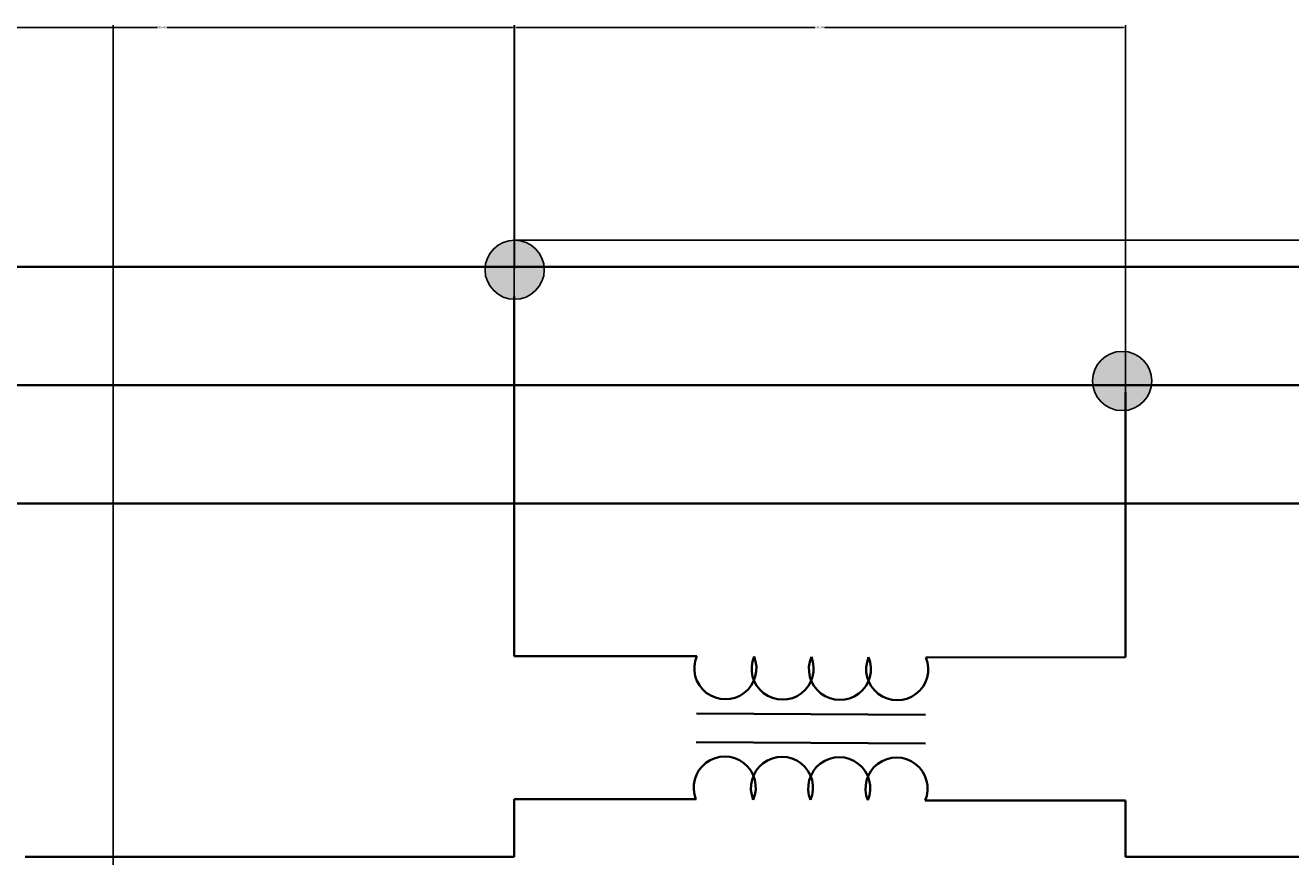
# Model space of a CAD drawing. Units: inches. Extents: x 738 to 1068, y 378 to 757.
# Tile 40 of 41: x 860 to 967, y 686 to 757. Entities that reach past the tile are written whole.
import ezdxf

# ---------------------------------------------------------------- set-up
doc = ezdxf.new("R2010")
doc.units = ezdxf.units.IN
doc.header["$MEASUREMENT"] = 0
for name, color, linetype, lineweight in [('A-ANNO-DIMS', 2, 'Continuous', 18), ('E-CONN', 7, 'Continuous', 25), ('E-CONN-PATT', 7, 'Continuous', 13), ('E-POWR-EQPM', 4, 'Continuous', 35), ('E-POWR-FEED', 7, 'Continuous', 35)]:
    doc.layers.add(name, color=color, linetype=linetype, lineweight=lineweight)
doc.styles.get("Standard").update_dxf_attribs({"font": 'arial.ttf'})
doc.dimstyles.get("Standard").update_dxf_attribs({"dimtxt": 0.18, "dimasz": 0.18, "dimexe": 0.18, "dimexo": 0.0625, "dimgap": 0.09, "dimtad": 0, "dimtih": 1, "dimtoh": 1, "dimdec": 4, "dimzin": 0, "dimdsep": 46, "dimtxsty": 'Standard', "dimcen": 0.09, "dimadec": 0, "dimazin": 0, "dimtfac": 1, "dimtdec": 4, "dimtofl": 0, "dimtmove": 0, "dimatfit": 3, "dimfxl": 1, "dimtolj": 1, "dimtzin": 0, "dimarcsym": 0})

# ---------------------------------------------------------------- blocks, each defined once
blk = doc.blocks.new('Transformer')
for p, q in [((0.1, 0), (0.1, 0.4)), ((0.15, 0.4), (0.15, 0))]:
    blk.add_line(p, q)
for centre, start, end in [((0.0208, 0.35), 247.3801, 112.6199), ((0.2292, 0.35), 67.3801, 292.6199), ((0.0208, 0.25), 247.3801, 112.6199), ((0.2292, 0.25), 67.3801, 292.6199), ((0.0208, 0.15), 247.3801, 112.6199), ((0.2292, 0.15), 67.3801, 292.6199), ((0.0208, 0.05), 247.3801, 112.6199), ((0.2292, 0.05), 67.3801, 292.6199)]:
    blk.add_arc(centre, 0.0542, start, end)
blk = doc.blocks.new('*D18')
at = {"layer": 'A-ANNO-DIMS', "color": 0, "lineweight": -2, "transparency": 16777216}
for p, q in [((901.52, 738.38), (1068.18, 738.38)), ((1068, 738.2), (1068, 569.17)), ((1068, 399.78), (1068, 568.8)), ((1023.84, 399.6), (1068.18, 399.6))]:
    blk.add_line(p, q, dxfattribs=at)
at = {"layer": 'A-ANNO-DIMS', "color": 0, "transparency": 16777216}
for points in [[(1067.97, 738.2), (1068.03, 738.2), (1068, 738.38)], [(1067.97, 399.78), (1068.03, 399.78), (1068, 399.6)]]:
    blk.add_solid(points, dxfattribs=at)
at = {"layer": 'Defpoints', "color": 0, "transparency": 16777216}
for p in [(901.46, 738.38), (1068, 738.38), (1023.78, 399.6)]:
    blk.add_point(p, dxfattribs=at)
at = {"layer": 'A-ANNO-DIMS', "color": 0, "transparency": 16777216, "insert": (1068, 568.99), "char_height": 0.18, "attachment_point": 5}
blk.add_mtext('\\A1;338.8', dxfattribs=at)
blk = doc.blocks.new('*D26')
at = {"layer": 'A-ANNO-DIMS', "color": 0, "lineweight": -2, "transparency": 16777216}
for p, q in [((816.01, 647.05), (816.01, 756.51)), ((816.19, 756.33), (841.41, 756.33)), ((867.42, 756.33), (842.2, 756.33)), ((867.6, 647.05), (867.6, 756.51))]:
    blk.add_line(p, q, dxfattribs=at)
at = {"layer": 'A-ANNO-DIMS', "color": 0, "transparency": 16777216}
for points in [[(816.19, 756.36), (816.19, 756.3), (816.01, 756.33)], [(867.42, 756.36), (867.42, 756.3), (867.6, 756.33)]]:
    blk.add_solid(points, dxfattribs=at)
at = {"layer": 'Defpoints', "color": 0, "transparency": 16777216}
for p in [(867.6, 756.33), (816.01, 646.99), (867.6, 646.99)]:
    blk.add_point(p, dxfattribs=at)
at = {"layer": 'A-ANNO-DIMS', "color": 0, "transparency": 16777216, "insert": (841.8, 756.33), "char_height": 0.18, "attachment_point": 5}
blk.add_mtext('\\A1;51.59', dxfattribs=at)
blk = doc.blocks.new('*D36')
at = {"layer": 'A-ANNO-DIMS', "color": 0, "lineweight": -2, "transparency": 16777216}
for p, q in [((901.43, 703.32), (901.43, 756.51)), ((901.61, 756.33), (926.82, 756.33)), ((952.82, 756.33), (927.61, 756.33)), ((953, 703.23), (953, 756.51))]:
    blk.add_line(p, q, dxfattribs=at)
at = {"layer": 'A-ANNO-DIMS', "color": 0, "transparency": 16777216}
for points in [[(901.61, 756.36), (901.61, 756.3), (901.43, 756.33)], [(952.82, 756.36), (952.82, 756.3), (953, 756.33)]]:
    blk.add_solid(points, dxfattribs=at)
at = {"layer": 'Defpoints', "color": 0, "transparency": 16777216}
for p in [(953, 756.33), (901.43, 703.26), (953, 703.17)]:
    blk.add_point(p, dxfattribs=at)
at = {"layer": 'A-ANNO-DIMS', "color": 0, "transparency": 16777216, "insert": (927.22, 756.33), "char_height": 0.18, "attachment_point": 5}
blk.add_mtext('\\A1;51.58', dxfattribs=at)
blk = doc.blocks.new('*D37')
at = {"layer": 'A-ANNO-DIMS', "color": 0, "lineweight": -2, "transparency": 16777216}
for p, q in [((841.98, 736.19), (841.98, 756.51)), ((842.16, 756.33), (871.33, 756.33)), ((901.28, 756.33), (872.12, 756.33)), ((901.46, 735.94), (901.46, 756.51))]:
    blk.add_line(p, q, dxfattribs=at)
at = {"layer": 'A-ANNO-DIMS', "color": 0, "transparency": 16777216}
for points in [[(842.16, 756.36), (842.16, 756.3), (841.98, 756.33)], [(901.28, 756.36), (901.28, 756.3), (901.46, 756.33)]]:
    blk.add_solid(points, dxfattribs=at)
at = {"layer": 'Defpoints', "color": 0, "transparency": 16777216}
for p in [(901.46, 756.33), (841.98, 736.13), (901.46, 735.88)]:
    blk.add_point(p, dxfattribs=at)
at = {"layer": 'A-ANNO-DIMS', "color": 0, "transparency": 16777216, "insert": (871.72, 756.33), "char_height": 0.18, "attachment_point": 5}
blk.add_mtext('\\A1;59.48', dxfattribs=at)

msp = doc.modelspace()

# ---------------------------------------------------------------- hatches: boundary and pattern name
at = {"layer": 'E-CONN-PATT'}
h = msp.add_hatch(color=256, dxfattribs=at)
h.dxf.hatch_style = 1
h.paths.add_polyline_path([(898.9751, 736.1282), (903.9494, 736.1282, 0.90338626)])
h.paths.add_polyline_path([(903.9622, 735.8751, 0.02536311), (903.9494, 736.1282), (898.9751, 736.1282, 0.02536311), (898.9622, 735.8751, 1)])
h.paths.add_polyline_path([(950.221, 726.4817, 0.0354864), (950.2461, 726.1282), (955.1958, 726.1282, 0.0354864), (955.221, 726.4817, 1)])
h.paths.add_polyline_path([(955.1958, 726.1282), (950.2461, 726.1282, 0.86730505)])

# ---------------------------------------------------------------- linework, layer by layer
at = {"layer": 'E-CONN'}
for points in [[(898.9622, 735.8751, 1), (903.9622, 735.8751, 1)], [(950.221, 726.4817, 1), (955.221, 726.4817, 1)]]:
    msp.add_lwpolyline(points, format="xyb", close=True, dxfattribs=at)
at = {"layer": 'E-POWR-EQPM'}
msp.add_line((921.6695, 703.2129), (921.6575, 703.2129), dxfattribs=at)
at = {"layer": 'E-POWR-FEED'}
for p, q in [((841.9816, 736.1282), (1012.7462, 736.1282)), ((901.4286, 733.6278), (901.4286, 703.2602)), ((841.9816, 726.1282), (1012.7462, 726.1282)), ((953.0038, 703.1664), (953.0038, 725.5434)), ((841.9816, 716.1282), (1012.7462, 716.1282)), ((916.8305, 703.2545), (901.4286, 703.2602)), ((936.1627, 703.1462), (953.0038, 703.1664)), ((916.7629, 691.1719), (901.4286, 691.1719)), ((901.4286, 691.1719), (901.4286, 686.3292)), ((936.095, 691.0636), (953.0038, 691.0636)), ((953.0038, 691.0636), (953.0038, 686.3292)), ((901.4286, 686.3292), (860.1747, 686.3292)), ((953.0038, 686.3292), (1023.824, 686.3292))]:
    msp.add_line(p, q, dxfattribs=at)

# ---------------------------------------------------------------- block references
at = {"layer": 'E-POWR-EQPM', "xscale": 48.33110256232303, "yscale": 48.33110256232303, "zscale": 48.33110256232303, "rotation": 89.67916066502065}
msp.add_blockref('Transformer', (936.095, 691.0636), dxfattribs=at)

# ---------------------------------------------------------------- dimensions: what is measured, and where the dimension line sits
at = {"layer": 'A-ANNO-DIMS'}
for base, p1, p2, picture, middle in [((867.5964, 756.3251), (816.0076, 646.9853), (867.5964, 646.9853), '*D26', (841.802, 756.3251)), ((901.4622, 756.3251), (841.9816, 736.1282), (901.4622, 735.8751), '*D37', (871.7219, 756.3251)), ((953.0038, 756.3251), (901.4286, 703.2602), (953.0038, 703.1664), '*D36', (927.2162, 756.3251))]:
    dim = msp.add_linear_dim(base=base, p1=p1, p2=p2, dimstyle='Standard', override={"dimdec": 2, "dimlfac": 1, "dimrnd": 0, "dimzin": 0, "dimdsep": 46, "dimlunit": 2}, dxfattribs=at)
    dim.commit()
    dim.dimension.update_dxf_attribs({"geometry": picture, "text_midpoint": middle})
dim = msp.add_linear_dim(base=(1067.9992, 738.3751), p1=(1023.779, 399.5952), p2=(901.4622, 738.3751), angle=90, dimstyle='Standard', override={"dimdec": 1, "dimlfac": 1, "dimrnd": 0, "dimzin": 0, "dimdsep": 46, "dimlunit": 2}, dxfattribs=at)
dim.commit()
dim.dimension.update_dxf_attribs({"geometry": '*D18', "text_midpoint": (1067.9992, 568.9851)})

doc.saveas('drawing.dxf')
